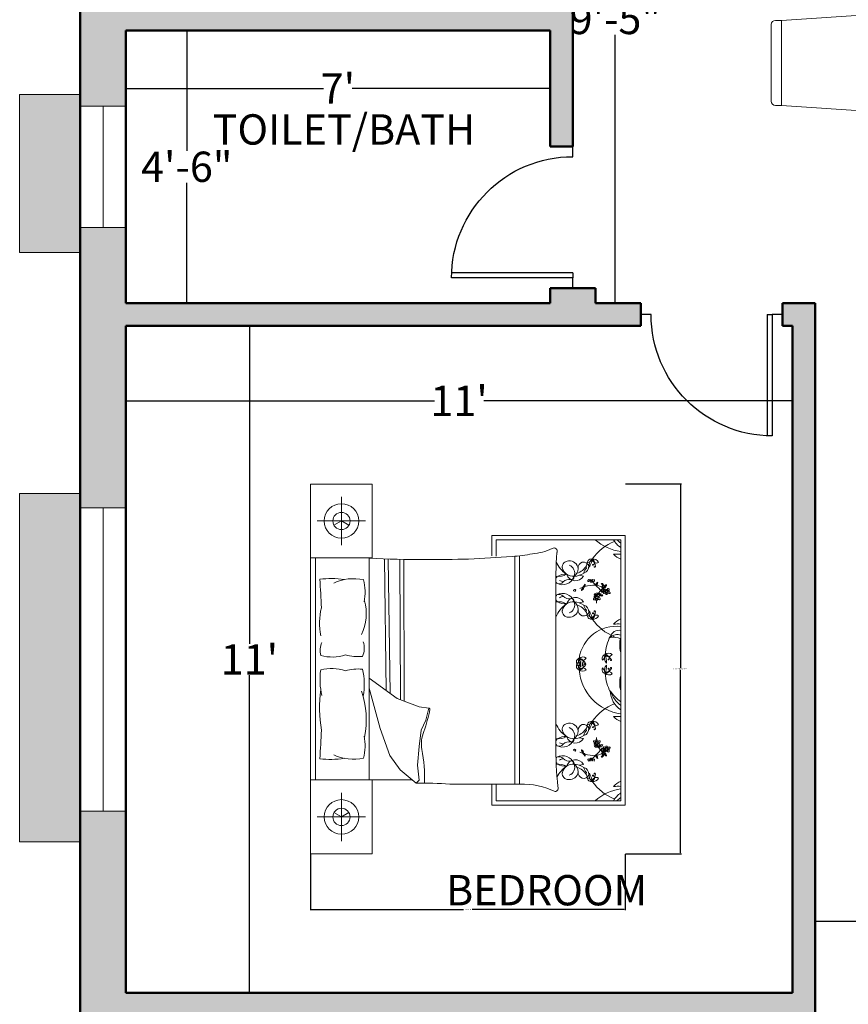
# Model space of a CAD drawing. Units: inches. Extents: x -28 to 544, y -640 to 52.
# Tile 4 of 11: x 5 to 169, y -389 to -194. Entities that reach past the tile are written whole.
import ezdxf

# ---------------------------------------------------------------- set-up
doc = ezdxf.new("R2010")
doc.units = ezdxf.units.IN
doc.header["$MEASUREMENT"] = 0
for name, color, linetype, lineweight in [('A-ANNO-DIMS', 2, 'Continuous', 18), ('A-AREA-IDEN', 7, 'Continuous', 25), ('A-DOOR', 3, 'Continuous', 25), ('A-FURN', 8, 'Continuous', 18), ('A-GLAZ', 4, 'Continuous', 20), ('A-ROOF', 8, 'Continuous', 18), ('A-ROOF-PATT', 252, 'Continuous', 13), ('A-WALL', 7, 'Continuous', 50), ('A-WALL-PATT', 5, 'Continuous', 13)]:
    doc.layers.add(name, color=color, linetype=linetype, lineweight=lineweight)
doc.styles.get("Standard").update_dxf_attribs({"font": 'arial.ttf'})
doc.dimstyles.get("Standard").update_dxf_attribs({"dimtxt": 0.18, "dimasz": 0.18, "dimexe": 0.18, "dimexo": 0.0625, "dimgap": 0.09, "dimtad": 0, "dimtih": 1, "dimtoh": 1, "dimdec": 0, "dimzin": 0, "dimdsep": 46, "dimlunit": 3, "dimtxsty": 'Standard', "dimcen": 0.09, "dimadec": 0, "dimazin": 0, "dimtfac": 1, "dimtdec": 0, "dimtofl": 0, "dimtmove": 0, "dimatfit": 3, "dimfxl": 1, "dimtolj": 1, "dimtzin": 0, "dimarcsym": 0})

# ---------------------------------------------------------------- blocks, each defined once
blk = doc.blocks.new('*D13')
at = {"layer": 'A-ANNO-DIMS', "color": 0, "lineweight": -2, "transparency": 16777216}
for p, q in [((38.26, -196.24), (37.84, -196.24)), ((38.02, -196.42), (38.02, -220.09)), ((38.02, -250.06), (38.02, -226.39)), ((43.05, -250.24), (37.84, -250.24))]:
    blk.add_line(p, q, dxfattribs=at)
at = {"layer": 'A-ANNO-DIMS', "color": 0, "transparency": 16777216}
for points in [[(37.99, -196.42), (38.05, -196.42), (38.02, -196.24)], [(37.99, -250.06), (38.05, -250.06), (38.02, -250.24)]]:
    blk.add_solid(points, dxfattribs=at)
at = {"layer": 'Defpoints', "color": 0, "transparency": 16777216}
for p in [(38.32, -196.24), (38.02, -250.24), (43.11, -250.24)]:
    blk.add_point(p, dxfattribs=at)
at = {"layer": 'A-ANNO-DIMS', "color": 0, "transparency": 16777216, "insert": (38.02, -223.24), "char_height": 6, "attachment_point": 5}
blk.add_mtext('\\A1;4\'-6"', dxfattribs=at)
blk = doc.blocks.new('*D14')
at = {"layer": 'A-ANNO-DIMS', "color": 0, "lineweight": -2, "transparency": 16777216}
for p, q in [((25.94, -207.68), (25.94, -207.56)), ((26.12, -207.74), (65.12, -207.74)), ((109.76, -207.74), (70.77, -207.74)), ((109.94, -207.68), (109.94, -207.56))]:
    blk.add_line(p, q, dxfattribs=at)
at = {"layer": 'A-ANNO-DIMS', "color": 0, "transparency": 16777216}
for points in [[(26.12, -207.71), (26.12, -207.77), (25.94, -207.74)], [(109.76, -207.71), (109.76, -207.77), (109.94, -207.74)]]:
    blk.add_solid(points, dxfattribs=at)
at = {"layer": 'Defpoints', "color": 0, "transparency": 16777216}
for p in [(25.94, -207.74), (25.94, -207.74), (109.94, -207.74)]:
    blk.add_point(p, dxfattribs=at)
at = {"layer": 'A-ANNO-DIMS', "color": 0, "transparency": 16777216, "insert": (67.94, -207.74), "char_height": 6, "attachment_point": 5}
blk.add_mtext("\\A1;7'", dxfattribs=at)
blk = doc.blocks.new('*D15')
at = {"layer": 'A-ANNO-DIMS', "color": 0, "lineweight": -2, "transparency": 16777216}
for p, q in [((50.43, -254.92), (50.43, -317.64)), ((50.5, -254.74), (50.61, -254.74)), ((50.43, -386.56), (50.43, -323.84)), ((50.5, -386.74), (50.61, -386.74))]:
    blk.add_line(p, q, dxfattribs=at)
at = {"layer": 'A-ANNO-DIMS', "color": 0, "transparency": 16777216}
for points in [[(50.4, -254.92), (50.46, -254.92), (50.43, -254.74)], [(50.4, -386.56), (50.46, -386.56), (50.43, -386.74)]]:
    blk.add_solid(points, dxfattribs=at)
at = {"layer": 'Defpoints', "color": 0, "transparency": 16777216}
for p in [(50.43, -254.74), (50.43, -386.74), (50.43, -386.74)]:
    blk.add_point(p, dxfattribs=at)
at = {"layer": 'A-ANNO-DIMS', "color": 0, "transparency": 16777216, "insert": (50.43, -320.74), "char_height": 6, "attachment_point": 5}
blk.add_mtext("\\A1;11'", dxfattribs=at)
blk = doc.blocks.new('*D16')
at = {"layer": 'A-ANNO-DIMS', "color": 0, "lineweight": -2, "transparency": 16777216}
for p, q in [((25.94, -269.5), (25.94, -269.38)), ((26.12, -269.56), (87.05, -269.56)), ((157.76, -269.56), (96.84, -269.56)), ((157.94, -269.5), (157.94, -269.38))]:
    blk.add_line(p, q, dxfattribs=at)
at = {"layer": 'A-ANNO-DIMS', "color": 0, "transparency": 16777216}
for points in [[(26.12, -269.53), (26.12, -269.59), (25.94, -269.56)], [(157.76, -269.53), (157.76, -269.59), (157.94, -269.56)]]:
    blk.add_solid(points, dxfattribs=at)
at = {"layer": 'Defpoints', "color": 0, "transparency": 16777216}
for p in [(25.94, -269.56), (25.94, -269.56), (157.94, -269.56)]:
    blk.add_point(p, dxfattribs=at)
at = {"layer": 'A-ANNO-DIMS', "color": 0, "transparency": 16777216, "insert": (91.94, -269.56), "char_height": 6, "attachment_point": 5}
blk.add_mtext("\\A1;11'", dxfattribs=at)
blk = doc.blocks.new('*D35')
at = {"layer": 'A-ANNO-DIMS', "color": 0, "lineweight": -2, "transparency": 16777216}
for p, q in [((126.88, -137.74), (122.68, -137.74)), ((122.86, -137.92), (122.86, -190.84)), ((122.86, -250.06), (122.86, -197.14)), ((127.88, -250.24), (122.68, -250.24))]:
    blk.add_line(p, q, dxfattribs=at)
at = {"layer": 'A-ANNO-DIMS', "color": 0, "transparency": 16777216}
for points in [[(122.83, -137.92), (122.89, -137.92), (122.86, -137.74)], [(122.83, -250.06), (122.89, -250.06), (122.86, -250.24)]]:
    blk.add_solid(points, dxfattribs=at)
at = {"layer": 'Defpoints', "color": 0, "transparency": 16777216}
for p in [(126.94, -137.74), (122.86, -250.24), (127.94, -250.24)]:
    blk.add_point(p, dxfattribs=at)
at = {"layer": 'A-ANNO-DIMS', "color": 0, "transparency": 16777216, "insert": (122.86, -193.99), "char_height": 6, "attachment_point": 5}
blk.add_mtext('\\A1;9\'-5"', dxfattribs=at)
blk = doc.blocks.new('*D39')
at = {"layer": 'A-ANNO-DIMS', "color": 0, "lineweight": -2, "transparency": 16777216}
for p, q in [((162.44, -377.5), (162.44, -372.33)), ((162.62, -372.51), (201.62, -372.51)), ((246.26, -372.51), (207.27, -372.51)), ((246.44, -377.5), (246.44, -372.33))]:
    blk.add_line(p, q, dxfattribs=at)
at = {"layer": 'A-ANNO-DIMS', "color": 0, "transparency": 16777216}
for points in [[(162.62, -372.48), (162.62, -372.54), (162.44, -372.51)], [(246.26, -372.48), (246.26, -372.54), (246.44, -372.51)]]:
    blk.add_solid(points, dxfattribs=at)
at = {"layer": 'Defpoints', "color": 0, "transparency": 16777216}
for p in [(246.44, -372.51), (162.44, -377.56), (246.44, -377.56)]:
    blk.add_point(p, dxfattribs=at)
at = {"layer": 'A-ANNO-DIMS', "color": 0, "transparency": 16777216, "insert": (204.44, -372.51), "char_height": 6, "attachment_point": 5}
blk.add_mtext("\\A1;7'", dxfattribs=at)
blk = doc.blocks.new('BED-DOUBLE-HEADBOARD-73')
for p, q in [((0, 0), (0, 73.21)), ((6.1, 61.11), (6.1, 70.67)), ((10.88, 65.89), (1.32, 65.89)), ((35.89, 58.98), (35.89, 63.04)), ((35.89, 63.04), (62.26, 63.04)), ((62.26, 63.04), (62.26, 9.66)), ((36.74, 62.19), (36.74, 58.96)), ((61.41, 62.19), (36.74, 62.19)), ((61.41, 10.51), (61.41, 62.19)), ((0.94, 58.57), (0.94, 14.64)), ((11.57, 14.64), (11.57, 58.57)), ((40.45, 58.9), (40.45, 13.8)), ((41.37, 58.97), (41.37, 13.8)), ((14.61, 58.37), (14.98, 32.31)), ((15.36, 58.34), (15.74, 31.76)), ((17.67, 58.31), (17.78, 30.51)), ((18.42, 58.31), (18.53, 30.22)), ((53.99, 54.97), (53.16, 55.14)), ((48.56, 51.47), (48.56, 21.74)), ((53.99, 49.86), (53.16, 49.7)), ((11.57, 34.76), (17.15, 30.74)), ((13.75, 24.81), (11.57, 32.8)), ((17.15, 30.74), (21.45, 29.11)), ((21.45, 29.11), (23.38, 28.82)), ((23.38, 28.82), (22.79, 26.44)), ((22.79, 26.44), (21.9, 24.52)), ((15.67, 19.47), (13.75, 24.81)), ((21.9, 24.52), (21.45, 21.25)), ((53.99, 22.84), (53.16, 23)), ((21.45, 21.25), (21.15, 17.55)), ((17.75, 16.66), (15.67, 19.47)), ((21.15, 17.55), (21.45, 14.58)), ((53.99, 17.73), (53.16, 17.56)), ((20.86, 13.99), (17.75, 16.66)), ((0, 14.64), (20.09, 14.64)), ((21.45, 14.58), (20.86, 13.99)), ((35.89, 9.66), (35.89, 13.8)), ((36.74, 13.8), (36.74, 10.51)), ((6.1, 12.1), (6.1, 2.54)), ((36.74, 10.51), (61.41, 10.51)), ((62.26, 9.66), (35.89, 9.66)), ((10.88, 7.32), (1.32, 7.32))]:
    blk.add_line(p, q)
for points in [[(0, 58.57), (12.2, 58.57), (12.2, 73.21), (0, 73.21)], [(6.1, 65.89), (4.62, 65.04)], [(6.1, 65.89), (7.58, 65.04)], [(12.2, 14.64), (12.2, 0), (0, 0)], [(6.1, 7.32), (4.62, 8.18)], [(6.1, 7.32), (7.58, 8.18)]]:
    blk.add_lwpolyline(points)
for points in [[(39.88, 58.88, 0.056112), (43.91, 59.41, 0.095341), (47.79, 60.44)], [(1.82, 54.36, -0.074897), (6.61, 54.28, 0.472817)], [(6.87, 39.39, -0.14099), (2, 39.24, -0.235245)], [(6.87, 36.26, 0.14099), (2, 36.41, 0.235245)], [(1.82, 18.85, 0.074897), (6.61, 18.94, -0.472817)], [(27.56, 13.83, 0.001242), (41.45, 13.8, -0.127202), (48.38, 12.33)]]:
    blk.add_lwpolyline(points, format="xyb")
for centre, radius in [((6.1, 65.89), 3.42), ((6.1, 65.89), 1.71), ((56.64, 50.74), 0.186), ((58.61, 51.96), 0.186), ((56.64, 21.96), 0.186), ((58.61, 20.74), 0.186), ((6.1, 7.32), 3.42), ((6.1, 7.32), 1.71)]:
    blk.add_circle(centre, radius)
for centre, radius, start, end in [((48.16, 59.89), 0.667, 336.5219, 123.8264), ((63.65, 52.95), 9.56, 111.4092, 145.6135), ((62.7, 69.31), 9.56, 228.1144, 262.255), ((63.98, 64.51), 4.66, 209.8884, 236.5383), ((64.85, 66.19), 5.81, 223.5186, 233.6964), ((20.52, 189.81), 131.55, 266.1, 270.9282), ((25.3, 229.86), 171.6, 269.1145, 274.8735), ((119.76, 53.71), 71.24, 175.2402, 181.8035), ((62.9, 61.9), 3.89, 221.0454, 247.4453), ((60.81, 72.55), 13.23, 266.3481, 272.5919), ((53.71, 59.98), 5.54, 203.6453, 236.3329), ((51.05, 56.75), 1.24, 88.9462, 185.5144), ((51.97, 57.13), 2.2, 193.079, 274.7067), ((51.23, 56.25), 1.75, 7.1143, 95.0551), ((50.57, 55.56), 1.7, 338.5779, 68.4181), ((51.63, 58.83), 3.46, 288.2955, 328.7386), ((54.05, 56.65), 1.1, 19.1312, 189.736), ((53.72, 56.91), 1.37, 285.6955, 4.031), ((55.54, 55.43), 1.46, 128.4175, 173.8338), ((55.24, 56.88), 0.673, 126.7319, 206.0245), ((55.57, 57.58), 0.793, 76.272, 177.0484), ((54.36, 59.2), 1.63, 284.7031, 328.6173), ((56.64, 57.12), 1.51, 125.7657, 194.5347), ((49.23, 59.8), 6.69, 332.8176, 347.4827), ((55.98, 57.31), 1.06, 20.9613, 102.2885), ((56.55, 58.37), 0.798, 181.7131, 301.5367), ((53.94, 56.76), 2.42, 2.0648, 41.1598), ((55.39, 57.66), 0.782, 316.2238, 62.3173), ((55.84, 57.2), 0.0623, 20.2667, 316.2271), ((56.17, 56.85), 0.0577, 52.0591, 168.5166), ((56.23, 56.84), 0.119, 168.5166, 2.0648), ((49.1, 57.95), 3.03, 259.249, 301.1782), ((49.37, 54.19), 0.882, 127.675, 162.5814), ((49.89, 55.6), 2.33, 240.8249, 340.7178), ((50.42, 52.56), 2.82, 85.2696, 124.215), ((52.41, 55.88), 1.82, 196.8663, 330.0915), ((51.65, 54.73), 0.454, 254.8529, 12.6959), ((50.42, 52.56), 2.82, 53.6555, 57.2989), ((50.84, 56.55), 2.13, 305.9599, 357.6409), ((51.91, 58.86), 3.93, 273.4924, 303.7117), ((-694.9, 14.01), 697.9, 2.85022, 3.31479), ((8.53, 45.04), 9.44, 78.2417, 114.8684), ((0.97, 51.75), 9.81, 348.9631, 14.8961), ((49.37, 54.19), 0.882, 196.6343, 225.5483), ((49.19, 54.56), 1.1, 246.1646, 318.4347), ((50.31, 55.95), 2.1, 240.0851, 262.564), ((51.14, 52.84), 1.5, 74.8529, 138.4347), ((56.02, 47.13), 6.06, 110.1059, 116.9968), ((53.95, 52.6), 0.149, 83.9457, 185.6216), ((53.35, 52.74), 0.614, 328.836, 0.8141), ((53.67, 52.56), 0.351, 306.5232, 32.4668), ((54.09, 52.83), 0.149, 112.5583, 214.2343), ((53.99, 53.1), 0.351, 265.7131, 351.6568), ((53.68, 53.29), 0.614, 297.3659, 329.344), ((53.22, 53.82), 1.18, 313.6929, 321.7899), ((54.52, 53.01), 0.384, 115.5379, 168.6744), ((53.21, 53.57), 1.16, 329.344, 349.7412), ((56.02, 47.13), 6.06, 86.1723, 106.4158), ((52.29, 53.3), 2.06, 352.8698, 1.6736), ((55.02, 54.05), 0.144, 125.0752, 284.7644), ((55.25, 54.1), 0.311, 127.3642, 168.4363), ((55, 54.35), 0.448, 277.4968, 341.2737), ((55.36, 54.14), 0.178, 88.1325, 178.8919), ((55.72, 53.95), 0.385, 136.3462, 189.6513), ((55.5, 53.92), 0.161, 189.6513, 312.3208), ((55.54, 54.36), 0.186, 183.2768, 356.7232), ((56.12, 54.03), 0.61, 164.2829, 186.9148), ((55.4, 54.02), 0.305, 312.3208, 40.2111), ((56.04, 54.37), 0.433, 201.6382, 274.947), ((55.47, 53.77), 0.566, 42.3896, 66.5724), ((61.18, 58.25), 6.95, 217.9541, 226.8459), ((55.88, 54.11), 0.308, 10.9597, 52.2379), ((56.07, 54.08), 0.143, 274.947, 37.5263), ((56.55, 53.27), 0.149, 112.5583, 214.2343), ((56.45, 53.53), 0.351, 265.7131, 351.6568), ((56.14, 53.73), 0.614, 297.3659, 329.344), ((56.17, 50.15), 3.04, 60.7959, 85.244), ((49.7, 45.78), 10, 37.8256, 47.7588), ((55.68, 54.25), 1.18, 313.6929, 321.7899), ((56.98, 53.45), 0.384, 115.5379, 168.6744), ((55.68, 54), 1.16, 329.344, 349.7412), ((54.75, 53.74), 2.06, 352.8698, 1.6736), ((60.21, 49.84), 3.65, 130.182, 149.456), ((57.66, 53.32), 0.208, 33.0979, 123.1364), ((53.07, 50.39), 5.45, 31.1156, 34.8118), ((57.35, 52.96), 0.564, 2.3172, 70.5201), ((57.08, 52.35), 0.85, 310.9365, 22.7695), ((57.82, 52.83), 0.163, 135.7354, 318.1297), ((57.55, 53.09), 0.216, 315.7354, 31.1156), ((57.37, 52.63), 0.5, 319.3812, 5.5456), ((57.94, 52.83), 0.163, 68.2452, 250.6395), ((57.57, 53.03), 0.485, 352.6008, 57.1845), ((59.3, 49.77), 3.25, 111.7087, 116.2181), ((56.17, 50.15), 3.04, 47.5083, 55.9967), ((58.03, 53.14), 0.485, 252.8042, 349.6943), ((57.57, 52.27), 0.517, 331.1838, 51.6792), ((58.08, 53.18), 0.216, 248.2452, 323.6254), ((57.89, 53.31), 0.564, 291.7087, 3.0299), ((53.87, 56.28), 5.45, 323.6254, 327.3216), ((58.34, 53.17), 0.208, 325.6077, 55.6462), ((49.37, 50.64), 0.882, 134.4517, 156.7144), ((49.89, 49.23), 2.33, 19.2822, 119.1751), ((49.19, 50.27), 1.1, 41.5653, 113.8354), ((50.31, 48.88), 2.1, 97.436, 119.9149), ((51.14, 51.99), 1.5, 221.5653, 285.1471), ((52.41, 48.95), 1.82, 29.9085, 163.1337), ((52.25, 52.22), 0.229, 169.5864, 349.5616), ((52.34, 52.21), 0.141, 349.5616, 167.2949), ((53.99, 52.13), 0.384, 129.5056, 182.6421), ((52.88, 53.02), 1.16, 308.4388, 328.836), ((52.68, 53.96), 2.06, 296.5064, 305.3102), ((52.67, 52.9), 1.18, 336.3901, 344.4871), ((56.35, 50.49), 0.311, 93.635, 168.4363), ((56.37, 52.17), 0.85, 253.6301, 325.4631), ((56.6, 50.99), 0.601, 82.0748, 142.6895), ((56.54, 51.82), 0.617, 228.342, 274.9894), ((56.31, 50.98), 0.183, 138.2946, 276.2474), ((56.38, 50.95), 0.254, 358.5719, 143.8954), ((56.47, 50.53), 0.178, 88.1325, 178.8919), ((56.53, 51.15), 0.257, 208.8493, 269.9355), ((56.31, 51.09), 0.293, 274.2123, 318.1587), ((56.56, 51.72), 0.517, 273.8774, 357.1501), ((57.21, 50.79), 0.588, 121.9501, 165.2442), ((56.76, 52.08), 0.5, 262.0748, 308.2393), ((56.8, 51.02), 0.123, 262.868, 7.094), ((56.58, 50.16), 0.566, 42.3896, 66.5724), ((56.79, 51.12), 0.368, 278.5614, 22.5914), ((56.99, 50.49), 0.308, 10.9597, 118.7804), ((60.21, 49.84), 3.65, 156.1523, 156.9499), ((56.99, 51.14), 0.185, 44.3732, 121.9501), ((57.56, 51.57), 0.517, 181.4625, 249.4747), ((57.48, 51.98), 0.5, 215.1128, 261.2773), ((57.88, 51.95), 0.85, 197.889, 269.722), ((57.61, 51.66), 0.617, 248.3627, 295.0101), ((57.31, 50.89), 0.601, 20.6625, 81.2773), ((58.2, 51.92), 0.601, 139.3812, 199.9959), ((57.47, 52.31), 0.617, 285.6484, 332.2957), ((58.1, 51.65), 0.144, 125.0752, 284.7644), ((58.32, 51.71), 0.311, 93.635, 168.4363), ((58.28, 52.2), 0.183, 138.2946, 276.2474), ((58.08, 51.96), 0.448, 277.4968, 341.2737), ((58.35, 52.17), 0.254, 358.5719, 143.8954), ((58.43, 51.75), 0.178, 88.1325, 178.8919), ((58.5, 52.37), 0.257, 208.8493, 269.9355), ((58.28, 52.31), 0.293, 274.2123, 318.1587), ((58.79, 51.56), 0.385, 136.3462, 189.6513), ((58.57, 51.52), 0.161, 189.6513, 312.3208), ((59.19, 51.63), 0.61, 164.2829, 186.9148), ((59.17, 52.01), 0.588, 121.9501, 165.2442), ((58.47, 51.63), 0.305, 312.3208, 40.2111), ((59.12, 51.97), 0.433, 201.6382, 274.947), ((58.77, 52.24), 0.123, 262.868, 7.094), ((58.54, 51.38), 0.566, 42.3896, 66.5724), ((58.75, 52.34), 0.368, 278.5614, 22.5914), ((58.95, 51.71), 0.308, 10.9597, 118.7804), ((58.96, 52.36), 0.185, 44.3732, 121.9501), ((59.14, 51.68), 0.143, 274.947, 37.5263), ((1.69, 47.52), 9.32, 333.8761, 16.1746), ((49.37, 50.64), 0.882, 203.2856, 232.325), ((49.1, 46.88), 3.03, 58.8218, 100.2867), ((53.71, 44.85), 5.54, 123.6671, 158.5059), ((50.42, 52.28), 2.82, 235.785, 274.7304), ((51.97, 47.7), 2.2, 85.2933, 166.921), ((50.57, 49.27), 1.7, 291.5819, 21.4221), ((51.65, 50.1), 0.454, 347.3041, 105.1471), ((50.42, 52.28), 2.82, 302.7011, 306.3445), ((50.84, 48.28), 2.13, 2.3591, 54.0401), ((51.91, 45.97), 3.93, 56.2883, 86.5076), ((51.63, 46), 3.46, 31.2614, 71.7045), ((55.54, 49.4), 1.46, 186.1662, 231.5825), ((53.72, 47.92), 1.37, 355.969, 74.3045), ((56.13, 50.43), 0.144, 125.0752, 284.7644), ((56.11, 50.74), 0.448, 277.4968, 341.2737), ((56.83, 50.34), 0.385, 136.3462, 189.6513), ((56.6, 50.3), 0.161, 189.6513, 312.3208), ((60.21, 49.84), 3.65, 175.2415, 182.8929), ((57.23, 50.41), 0.61, 164.2829, 186.9148), ((56.51, 50.41), 0.305, 312.3208, 40.2111), ((57.15, 50.75), 0.433, 201.6382, 274.947), ((57.18, 50.46), 0.143, 274.947, 37.5263), ((14.63, 45.68), 12.87, 166.3427, 191.1841), ((51.05, 48.08), 1.24, 174.4856, 271.0538), ((51.23, 48.59), 1.75, 264.9449, 352.8857), ((54.05, 48.18), 1.1, 170.264, 340.8688), ((55.24, 47.96), 0.673, 153.9755, 233.2681), ((55.57, 47.25), 0.793, 182.9516, 283.728), ((54.36, 45.63), 1.63, 31.3827, 75.2969), ((56.64, 47.71), 1.51, 165.4653, 234.2343), ((49.23, 45.03), 6.69, 12.5173, 27.1824), ((53.94, 48.07), 2.42, 318.8402, 357.9352), ((55.39, 47.18), 0.782, 297.6827, 43.7762), ((56.55, 46.46), 0.798, 58.4633, 178.2869), ((55.98, 47.52), 1.06, 257.7115, 339.0387), ((55.88, 47.64), 0.103, 43.7762, 339.7183), ((56.23, 47.99), 0.119, 357.9352, 191.4834), ((56.17, 47.98), 0.0577, 191.4834, 307.9409), ((60.49, 37.66), 7.4, 82.8636, 171.8197), ((63.65, 51.88), 9.56, 214.3865, 248.5908), ((62.9, 42.93), 3.89, 112.5547, 138.9546), ((60.81, 32.28), 13.23, 87.4081, 93.6519), ((67.82, 38.7), 9.56, 152.5854, 175.5377), ((61.01, 42.54), 1.72, 76.3898, 169.0739), ((60.77, 41.25), 2.17, 72.8609, 131.9049), ((59.82, 38.61), 4.28, 68.117, 96.6195), ((66.44, 41.37), 5.26, 162.9798, 196.4569), ((5.48, 40.25), 3.62, 153.3437, 196.1026), ((6.74, 40.74), 3.88, 335.0183, 18.5407), ((9.32, 48.02), 8.97, 254.1707, 275.9871), ((53.88, 37.92), 1.06, 50.8855, 132.2127), ((58.51, 38.68), 0.793, 106.1963, 206.9726), ((56.66, 39.48), 1.63, 314.6273, 358.5415), ((59.67, 38.82), 1.51, 155.6899, 224.4589), ((59, 38.66), 1.06, 50.8855, 132.2127), ((58.97, 39.86), 0.798, 211.6373, 331.4609), ((57.51, 37.15), 2.42, 31.989, 71.0841), ((51.91, 37.44), 6.69, 2.7418, 17.407), ((58.32, 38.66), 0.782, 346.148, 92.2415), ((69.15, 39.29), 7.77, 174.3643, 175.6213), ((74.47, 35.19), 13.89, 160.0972, 160.2783), ((53.39, 37.95), 0.793, 106.1963, 206.9726), ((53.39, 37.19), 0.793, 153.0274, 253.8037), ((51.54, 38.75), 1.63, 314.6273, 358.5415), ((51.54, 36.39), 1.63, 1.4585, 45.3727), ((54.55, 38.09), 1.51, 155.6899, 224.4589), ((54.55, 37.05), 1.51, 135.5411, 204.3101), ((53.85, 39.13), 0.798, 211.6373, 331.4609), ((53.2, 37.93), 0.782, 346.148, 92.2415), ((52.39, 36.42), 2.42, 31.989, 71.0841), ((46.79, 36.71), 6.69, 2.7418, 17.407), ((46.79, 38.43), 6.69, 342.593, 357.2582), ((52.39, 38.72), 2.42, 288.9159, 328.011), ((53.2, 37.21), 0.782, 267.7585, 13.852), ((53.82, 37.76), 0.0623, 50.1909, 346.0209), ((53.86, 37.38), 0.103, 13.852, 309.9245), ((54.34, 37.64), 0.119, 198.4408, 31.989), ((54.28, 37.62), 0.0577, 81.9833, 198.4408), ((54.34, 37.5), 0.119, 328.011, 161.5592), ((54.28, 37.52), 0.0577, 161.5592, 278.0167), ((59.67, 36.32), 1.51, 135.5411, 204.3101), ((51.91, 37.7), 6.69, 342.593, 357.2582), ((58.94, 38.49), 0.0623, 50.1909, 346.0209), ((59.46, 38.37), 0.119, 198.4408, 31.989), ((59.4, 38.35), 0.0577, 81.9833, 198.4408), ((14.9, 34.49), 13.05, 171.5249, 193.96), ((9.32, 27.63), 8.97, 84.0129, 105.8293), ((-2.29, 33.51), 12.91, 349.8617, 13.6238), ((53.85, 36.01), 0.798, 28.5391, 148.3627), ((53.88, 37.22), 1.06, 227.7873, 309.1145), ((62.7, 37.18), 9.56, 184.4623, 262.255), ((58.51, 36.46), 0.793, 153.0274, 253.8037), ((56.66, 35.66), 1.63, 1.4585, 45.3727), ((57.51, 37.99), 2.42, 288.9159, 328.011), ((58.32, 36.48), 0.782, 267.7585, 13.852), ((58.97, 35.28), 0.798, 28.5391, 148.3627), ((59, 36.48), 1.06, 227.7873, 309.1145), ((67.82, 36.44), 9.56, 184.4623, 207.4146), ((58.98, 36.64), 0.103, 13.852, 309.9245), ((59.46, 36.77), 0.119, 328.011, 161.5592), ((59.4, 36.79), 0.0577, 161.5592, 278.0167), ((66.44, 33.77), 5.26, 163.5431, 197.0202), ((69.15, 35.85), 7.77, 184.3787, 185.6357), ((74.47, 39.95), 13.89, 199.7217, 199.9028), ((28.32, 28.88), 26.55, 172.2196, 189.497), ((-6.01, 26.62), 17.02, 348.0397, 19.2615), ((63.98, 32.38), 4.66, 181.272, 236.5383), ((66.48, 37.11), 8.64, 214.0123, 234.053), ((64.85, 34.06), 5.81, 197.8504, 233.6964), ((63.65, 20.82), 9.56, 111.4092, 145.6135), ((-4.29, 33.9), 28.39, 340.1194, 349.3383), ((23.44, 28.65), 0.177, 358.8623, 109.7536), ((53.71, 27.85), 5.54, 201.4941, 236.3329), ((51.05, 24.62), 1.24, 88.9462, 185.5144), ((51.23, 24.12), 1.75, 7.1143, 95.0551), ((54.05, 24.52), 1.1, 19.1312, 189.736), ((55.57, 25.45), 0.793, 76.272, 177.0484), ((54.36, 27.07), 1.63, 284.7031, 328.6173), ((56.64, 24.99), 1.51, 125.7657, 194.5347), ((49.23, 27.67), 6.69, 332.8176, 347.4827), ((55.98, 25.18), 1.06, 20.9613, 102.2885), ((55.39, 25.53), 0.782, 316.2238, 62.3173), ((53.94, 24.63), 2.42, 2.0648, 41.1598), ((56.55, 26.24), 0.798, 181.7131, 301.5367), ((60.81, 40.42), 13.23, 266.3481, 272.5919), ((62.9, 29.77), 3.89, 221.0454, 247.4453), ((-694.9, 59.2), 697.9, 356.68521, 357.14978), ((27.87, 21.84), 5.96, 156.2616, 191.3392), ((51.97, 25), 2.2, 193.079, 274.7067), ((50.57, 23.43), 1.7, 338.5779, 68.4181), ((50.84, 24.42), 2.13, 305.9599, 357.6409), ((51.91, 26.73), 3.93, 273.4924, 303.7117), ((51.63, 26.7), 3.46, 288.2955, 328.7386), ((53.72, 24.78), 1.37, 285.6955, 4.031), ((55.54, 23.3), 1.46, 128.4175, 173.8338), ((55.24, 24.74), 0.673, 126.7319, 206.0245), ((55.84, 25.07), 0.0623, 20.2667, 316.2271), ((56.17, 24.72), 0.0577, 52.0591, 168.5166), ((56.23, 24.71), 0.119, 168.5166, 2.0648), ((0.97, 21.46), 9.81, 345.1039, 11.0369), ((124.77, 20.87), 76.21, 179.3433, 185.6887), ((49.1, 25.82), 3.03, 259.7133, 301.1782), ((49.37, 22.06), 0.882, 127.675, 156.7144), ((49.37, 22.06), 0.882, 203.229, 225.5483), ((49.89, 23.47), 2.33, 240.8249, 340.7178), ((49.19, 22.43), 1.1, 246.1646, 318.4347), ((50.42, 20.42), 2.82, 85.2696, 124.215), ((50.31, 23.82), 2.1, 240.0851, 262.564), ((51.14, 20.71), 1.5, 74.8529, 138.4347), ((52.41, 23.75), 1.82, 196.8663, 330.0915), ((51.65, 22.6), 0.454, 254.8529, 12.6959), ((50.42, 20.42), 2.82, 53.6555, 57.2989), ((56.13, 22.27), 0.144, 75.2356, 234.9248), ((56.35, 22.21), 0.311, 191.5637, 266.365), ((56.31, 21.72), 0.183, 83.7526, 221.7054), ((56.54, 20.88), 0.617, 85.0106, 131.658), ((56.11, 21.96), 0.448, 18.7263, 82.5032), ((56.38, 21.75), 0.254, 216.1046, 1.4281), ((56.47, 22.17), 0.178, 181.1081, 271.8675), ((56.53, 21.55), 0.257, 90.0645, 151.1507), ((56.31, 21.61), 0.293, 41.8413, 85.7877), ((56.83, 22.36), 0.385, 170.3487, 223.6538), ((56.6, 22.4), 0.161, 47.6792, 170.3487), ((60.21, 22.86), 3.65, 177.1071, 184.7585), ((56.56, 20.98), 0.517, 2.8499, 86.1226), ((57.23, 22.29), 0.61, 173.0852, 195.7171), ((57.21, 21.91), 0.588, 194.7558, 238.0499), ((56.51, 22.29), 0.305, 319.7889, 47.6792), ((57.15, 21.95), 0.433, 85.053, 158.3618), ((56.8, 21.68), 0.123, 352.906, 97.132), ((56.58, 22.54), 0.566, 293.4276, 317.6104), ((56.99, 22.21), 0.308, 241.2196, 349.0403), ((56.79, 21.58), 0.368, 337.4086, 81.4386), ((56.99, 21.56), 0.185, 238.0499, 315.6268), ((57.56, 21.13), 0.517, 110.5253, 178.5375), ((57.88, 20.75), 0.85, 90.278, 162.111), ((57.18, 22.24), 0.143, 322.4737, 85.053), ((57.61, 21.04), 0.617, 64.9899, 111.6373), ((57.31, 21.81), 0.601, 278.7227, 339.3375), ((8.53, 28.17), 9.44, 245.1316, 281.7583), ((-5.07, 15.24), 27.63, 357.4519, 11.3392), ((52.25, 20.48), 0.229, 10.4384, 190.4136), ((52.34, 20.49), 0.141, 192.7051, 10.4384), ((56.02, 25.57), 6.06, 243.0032, 249.8941), ((52.88, 19.68), 1.16, 31.164, 51.5612), ((53.99, 20.57), 0.384, 177.3579, 230.4944), ((52.68, 18.74), 2.06, 54.6898, 63.4936), ((52.67, 19.8), 1.18, 15.5129, 23.6099), ((53.95, 20.1), 0.149, 174.3784, 276.0543), ((53.35, 19.96), 0.614, 359.1859, 31.164), ((53.67, 20.14), 0.351, 327.5332, 53.4768), ((54.09, 19.87), 0.149, 145.7657, 247.4417), ((53.99, 19.61), 0.351, 8.3432, 94.2869), ((53.68, 19.41), 0.614, 30.656, 62.6341), ((53.22, 18.88), 1.18, 38.2101, 46.3071), ((54.52, 19.69), 0.384, 191.3256, 244.4621), ((53.21, 19.13), 1.16, 10.2588, 30.656), ((56.02, 25.57), 6.06, 253.5842, 273.8277), ((52.29, 19.4), 2.06, 358.3264, 7.1302), ((61.18, 14.45), 6.95, 133.1541, 142.0459), ((56.37, 20.53), 0.85, 34.5369, 106.3699), ((56.6, 21.71), 0.601, 217.3105, 277.9252), ((56.55, 19.44), 0.149, 145.7657, 247.4417), ((49.7, 26.92), 10, 312.2412, 322.1744), ((56.17, 22.55), 3.04, 274.756, 299.2041), ((56.45, 19.17), 0.351, 8.3432, 94.2869), ((56.14, 18.97), 0.614, 30.656, 62.6341), ((56.76, 20.62), 0.5, 51.7607, 97.9252), ((60.21, 22.86), 3.65, 203.0501, 203.8477), ((57.48, 20.72), 0.5, 98.7227, 144.8872), ((60.21, 22.86), 3.65, 210.544, 229.818), ((57.35, 19.74), 0.564, 289.4799, 357.6828), ((53.07, 22.32), 5.45, 325.1882, 328.8844), ((58.2, 20.78), 0.601, 160.0041, 220.6188), ((57.08, 20.35), 0.85, 337.2305, 49.0635), ((57.47, 20.4), 0.617, 27.7043, 74.3516), ((57.82, 19.88), 0.163, 41.8703, 224.2646), ((57.55, 19.61), 0.216, 328.8844, 44.2646), ((57.37, 20.07), 0.5, 354.4544, 40.6188), ((57.94, 19.87), 0.163, 109.3605, 291.7548), ((57.57, 19.67), 0.485, 302.8155, 7.3992), ((56.17, 22.55), 3.04, 304.0033, 312.4917), ((59.3, 22.93), 3.25, 243.7819, 248.2913), ((57.57, 20.43), 0.517, 308.3208, 28.8162), ((58.03, 19.56), 0.485, 10.3057, 107.1958), ((58.1, 21.05), 0.144, 75.2356, 234.9248), ((58.08, 19.52), 0.216, 36.3746, 111.7548), ((58.32, 20.99), 0.311, 191.5637, 266.365), ((58.28, 20.5), 0.183, 83.7526, 221.7054), ((57.89, 19.39), 0.564, 356.9701, 68.2913), ((58.08, 20.74), 0.448, 18.7263, 82.5032), ((58.35, 20.53), 0.254, 216.1046, 1.4281), ((58.43, 20.95), 0.178, 181.1081, 271.8675), ((53.87, 16.42), 5.45, 32.6784, 36.3746), ((58.5, 20.33), 0.257, 90.0645, 151.1507), ((58.28, 20.39), 0.293, 41.8413, 85.7877), ((58.79, 21.14), 0.385, 170.3487, 223.6538), ((58.57, 21.18), 0.161, 47.6792, 170.3487), ((58.34, 19.53), 0.208, 304.3538, 34.3923), ((59.19, 21.07), 0.61, 173.0852, 195.7171), ((59.17, 20.69), 0.588, 194.7558, 238.0499), ((58.47, 21.07), 0.305, 319.7889, 47.6792), ((59.12, 20.73), 0.433, 85.053, 158.3618), ((58.77, 20.46), 0.123, 352.906, 97.132), ((58.54, 21.32), 0.566, 293.4276, 317.6104), ((58.95, 20.99), 0.308, 241.2196, 349.0403), ((58.75, 20.36), 0.368, 337.4086, 81.4386), ((58.96, 20.34), 0.185, 238.0499, 315.6268), ((59.14, 21.02), 0.143, 322.4737, 85.053), ((49.37, 18.51), 0.882, 134.4517, 153.558), ((49.37, 18.51), 0.882, 210.0293, 232.325), ((49.1, 14.75), 3.03, 58.8218, 99.1554), ((49.89, 17.1), 2.33, 19.2822, 119.1751), ((49.19, 18.14), 1.1, 41.5653, 113.8354), ((50.42, 20.15), 2.82, 235.785, 274.7304), ((50.31, 16.75), 2.1, 97.436, 119.9149), ((51.97, 15.57), 2.2, 85.2933, 166.921), ((51.14, 19.86), 1.5, 221.5653, 285.1471), ((52.41, 16.82), 1.82, 29.9085, 163.1337), ((50.57, 17.14), 1.7, 291.5819, 21.4221), ((51.65, 17.97), 0.454, 347.3041, 105.1471), ((50.42, 20.15), 2.82, 302.7011, 306.3445), ((50.84, 16.15), 2.13, 2.3591, 54.0401), ((51.91, 13.84), 3.93, 56.2883, 86.5076), ((55.02, 18.65), 0.144, 75.2356, 234.9248), ((55.25, 18.6), 0.311, 191.5637, 232.6358), ((55, 18.35), 0.448, 18.7263, 82.5032), ((55.36, 18.56), 0.178, 181.1081, 271.8675), ((55.72, 18.75), 0.385, 170.3487, 223.6538), ((55.5, 18.79), 0.161, 47.6792, 170.3487), ((55.54, 18.34), 0.186, 3.2768, 176.7232), ((56.12, 18.67), 0.61, 173.0852, 195.7171), ((55.4, 18.68), 0.305, 319.7889, 47.6792), ((56.04, 18.34), 0.433, 85.053, 158.3618), ((55.47, 18.93), 0.566, 293.4276, 317.6104), ((55.88, 18.6), 0.308, 307.7621, 349.0403), ((56.07, 18.62), 0.143, 322.4737, 85.053), ((55.68, 18.45), 1.18, 38.2101, 46.3071), ((56.98, 19.25), 0.384, 191.3256, 244.4621), ((55.68, 18.7), 1.16, 10.2588, 30.656), ((54.75, 18.96), 2.06, 358.3264, 7.1302), ((57.66, 19.38), 0.208, 236.8636, 326.9021), ((53.71, 12.72), 5.54, 123.6671, 153.2997), ((51.05, 15.95), 1.24, 174.4856, 271.0538), ((51.23, 16.45), 1.75, 264.9449, 352.8857), ((51.63, 13.87), 3.46, 31.2614, 71.7045), ((54.05, 16.05), 1.1, 170.264, 340.8688), ((53.72, 15.79), 1.37, 355.969, 74.3045), ((55.54, 17.27), 1.46, 186.1662, 231.5825), ((55.24, 15.83), 0.673, 153.9755, 233.2681), ((56.64, 15.58), 1.51, 165.4653, 234.2343), ((49.23, 12.9), 6.69, 12.5173, 27.1824), ((53.94, 15.94), 2.42, 318.8402, 357.9352), ((55.88, 15.51), 0.103, 43.7762, 339.7183), ((56.23, 15.86), 0.119, 357.9352, 191.4834), ((56.17, 15.85), 0.0577, 191.4834, 307.9409), ((22.68, -53.14), 67.15, 85.8294, 91.553), ((54.36, 13.5), 1.63, 31.3827, 75.2969), ((55.57, 15.12), 0.793, 182.9516, 283.728), ((55.39, 15.04), 0.782, 297.6827, 43.7762), ((56.55, 14.33), 0.798, 58.4633, 178.2869), ((55.98, 15.39), 1.06, 257.7115, 339.0387), ((63.65, 19.75), 9.56, 214.3865, 248.5908), ((62.9, 10.8), 3.89, 112.5547, 138.9546), ((48.33, 13.01), 0.676, 273.98, 27.3412), ((62.7, 3.39), 9.56, 97.745, 131.8856), ((63.98, 8.19), 4.66, 123.4617, 150.1116), ((60.81, 0.15), 13.23, 87.4081, 93.6519), ((64.85, 6.51), 5.81, 126.3036, 136.4814)]:
    blk.add_arc(centre, radius, start, end)
blk = doc.blocks.new('DINING-SET-4')
for p, q in [((0.82, 49.45), (2.05, 49.45)), ((18.79, 50.59), (2.05, 49.45)), ((2.05, 32.63), (2.05, 49.45)), ((20.52, 48.95), (20.52, 33.13)), ((56.54, 48.95), (56.54, 33.13)), ((58.27, 50.59), (75.01, 49.45)), ((76.24, 49.45), (75.01, 49.45)), ((75.01, 32.63), (75.01, 49.45)), ((0, 33.45), (0, 48.63)), ((77.06, 33.45), (77.06, 48.63)), ((2.05, 32.63), (0.82, 32.63)), ((2.05, 32.63), (18.79, 31.49)), ((75.01, 32.63), (58.27, 31.49)), ((75.01, 32.63), (76.24, 32.63)), ((2.05, 22.09), (0.82, 22.09)), ((2.05, 22.09), (18.79, 23.23)), ((2.05, 22.09), (2.05, 5.27)), ((20.52, 5.77), (20.52, 21.59)), ((56.54, 5.77), (56.54, 21.59)), ((75.01, 22.09), (58.27, 23.23)), ((75.01, 22.09), (76.24, 22.09)), ((75.01, 22.09), (75.01, 5.27)), ((0, 21.27), (0, 6.09)), ((77.06, 21.27), (77.06, 6.09)), ((0.82, 5.27), (2.05, 5.27)), ((18.79, 4.13), (2.05, 5.27)), ((58.27, 4.13), (75.01, 5.27)), ((76.24, 5.27), (75.01, 5.27))]:
    blk.add_line(p, q)
for points in [[(55.63, 0), (21.43, 0), (21.43, 54.72), (55.63, 54.72)], [(53.35, 2.28), (23.71, 2.28), (23.71, 52.44), (53.35, 52.44)]]:
    blk.add_lwpolyline(points, close=True)
for centre, radius, start, end in [((0.82, 48.63), 0.821, 90, 180), ((18.88, 48.95), 1.64, 0, 93.1221), ((58.18, 48.95), 1.64, 86.8779, 180), ((76.24, 48.63), 0.821, 0, 90), ((0.82, 33.45), 0.821, 180, 270), ((18.88, 33.13), 1.64, 266.8779, 0), ((58.18, 33.13), 1.64, 180, 273.1221), ((76.24, 33.45), 0.821, 270, 0), ((0.82, 21.27), 0.821, 90, 180), ((18.88, 21.59), 1.64, 0, 93.1221), ((58.18, 21.59), 1.64, 86.8779, 180), ((76.24, 21.27), 0.821, 0, 90), ((0.82, 6.09), 0.821, 180, 270), ((76.24, 6.09), 0.821, 270, 0), ((18.88, 5.77), 1.64, 266.8779, 0), ((58.18, 5.77), 1.64, 180, 273.1221)]:
    blk.add_arc(centre, radius, start, end)
blk = doc.blocks.new('WIN-60IN')
for p, q in [((0, 9), (60, 9)), ((0, 0), (0, 9)), ((60, 9), (60, 0)), ((0, 4.5), (60, 4.5)), ((60, 0), (0, 0))]:
    blk.add_line(p, q)
blk = doc.blocks.new('WIN-24IN')
for p, q in [((0, 0), (0, 24)), ((0, 24), (9, 24)), ((4.5, 0), (4.5, 24)), ((9, 24), (9, 0)), ((9, 0), (0, 0))]:
    blk.add_line(p, q)
blk = doc.blocks.new('DOOR-SWING-24IN')
for p, q in [((25, 0), (25, 24)), ((26, 0), (26, 24)), ((2, 0), (0, 0)), ((25, 0), (26, 0)), ((28, 0), (26, 0))]:
    blk.add_line(p, q)
blk.add_arc((26, 0), 24, 90, 180)
blk = doc.blocks.new('*D67')
at = {"layer": 'A-ANNO-DIMS', "color": 0, "lineweight": -2, "transparency": 16777216}
for p, q in [((124.87, -286.01), (135.97, -286.01)), ((135.79, -286.19), (135.79, -322.44)), ((135.79, -359.04), (135.79, -322.8)), ((124.87, -359.22), (135.97, -359.22))]:
    blk.add_line(p, q, dxfattribs=at)
at = {"layer": 'A-ANNO-DIMS', "color": 0, "transparency": 16777216}
for points in [[(135.76, -286.19), (135.82, -286.19), (135.79, -286.01)], [(135.76, -359.04), (135.82, -359.04), (135.79, -359.22)]]:
    blk.add_solid(points, dxfattribs=at)
at = {"layer": 'Defpoints', "color": 0, "transparency": 16777216}
for p in [(124.81, -286.01), (135.79, -286.01), (124.81, -359.22)]:
    blk.add_point(p, dxfattribs=at)
at = {"layer": 'A-ANNO-DIMS', "color": 0, "transparency": 16777216, "insert": (135.79, -322.62), "char_height": 0.18, "attachment_point": 5}
blk.add_mtext('\\A1;DOUBLE BED B 6\'-1" TYP.', dxfattribs=at)
blk = doc.blocks.new('*D68')
at = {"layer": 'A-ANNO-DIMS', "color": 0, "lineweight": -2, "transparency": 16777216}
for p, q in [((62.55, -359.29), (62.55, -370.39)), ((124.81, -359.29), (124.81, -370.39)), ((62.73, -370.21), (92.83, -370.21)), ((124.63, -370.21), (94.53, -370.21))]:
    blk.add_line(p, q, dxfattribs=at)
at = {"layer": 'A-ANNO-DIMS', "color": 0, "transparency": 16777216}
for points in [[(62.73, -370.18), (62.73, -370.24), (62.55, -370.21)], [(124.63, -370.18), (124.63, -370.24), (124.81, -370.21)]]:
    blk.add_solid(points, dxfattribs=at)
at = {"layer": 'Defpoints', "color": 0, "transparency": 16777216}
for p in [(62.55, -359.22), (124.81, -359.22), (124.81, -370.21)]:
    blk.add_point(p, dxfattribs=at)
at = {"layer": 'A-ANNO-DIMS', "color": 0, "transparency": 16777216, "insert": (93.68, -370.21), "char_height": 0.18, "attachment_point": 5}
blk.add_mtext('\\A1;5\'-2 1/2" TYP.', dxfattribs=at)

msp = doc.modelspace()

# ---------------------------------------------------------------- hatches: boundary and pattern name
at = {"layer": 'A-ROOF-PATT'}
h = msp.add_hatch(color=256, dxfattribs=at)
h.dxf.hatch_style = 1
h.set_gradient(color1=(241, 235, 31), color2=(248, 153, 30))
h.paths.add_polyline_path([(124.53, 19.76), (58.75, 19.76), (58.75, 7.76), (124.53, 7.76)])
h.paths.add_polyline_path([(226.33, 19.76), (182.83, 19.76), (182.83, 7.76), (226.33, 7.76)])
h.paths.add_polyline_path([(313.67, 19.76), (271.84, 19.76), (271.84, 7.76), (313.67, 7.76)])
h.paths.add_polyline_path([(440.55, 19.76), (372.16, 19.76), (372.16, 7.76), (440.55, 7.76)])
h.paths.add_polyline_path([(492.44, -34.91), (480.44, -34.91), (480.44, -100.18), (492.44, -100.18)])
h.paths.add_polyline_path([(492.44, -151.37), (480.44, -151.37), (480.44, -179.02), (492.44, -179.02)])
h.paths.add_polyline_path([(492.44, -207.96), (480.44, -207.96), (480.44, -238.77), (492.44, -238.77)])
h.paths.add_polyline_path([(492.44, -289.99), (480.44, -289.99), (480.44, -354.53), (492.44, -354.53)])
h.paths.add_polyline_path([(492.44, -399.27), (480.44, -399.27), (480.44, -430), (492.44, -430)])
h.paths.add_polyline_path([(492.44, -475.99), (480.44, -475.99), (480.44, -546.14), (492.44, -546.14)])
h.paths.add_polyline_path([(442.7, -587.74), (368.43, -587.74), (368.43, -599.74), (442.7, -599.74)])
h.paths.add_polyline_path([(127.64, -587.74), (54.75, -587.74), (54.75, -599.74), (127.64, -599.74)])
h.paths.add_polyline_path([(16.94, -477.43), (4.94, -477.43), (4.94, -547.54), (16.94, -547.54)])
h.paths.add_polyline_path([(16.94, -399.8), (4.94, -399.8), (4.94, -430.58), (16.94, -430.58)])
h.paths.add_polyline_path([(16.94, -287.93), (4.94, -287.93), (4.94, -356.82), (16.94, -356.82)])
h.paths.add_polyline_path([(16.94, -208.93), (4.94, -208.93), (4.94, -240.18), (16.94, -240.18)])
h.paths.add_polyline_path([(16.94, -150), (4.94, -150), (4.94, -180.17), (16.94, -180.17)])
h.paths.add_polyline_path([(16.94, -32.89), (4.94, -32.89), (4.94, -101.73), (16.94, -101.73)])
at = {"layer": 'A-WALL-PATT'}
h = msp.add_hatch(color=256, dxfattribs=at)
h.dxf.hatch_style = 1
h.paths.add_polyline_path([(25.94, -235.24), (16.94, -235.24), (16.94, -290.74), (25.94, -290.74), (25.94, -254.74), (127.94, -254.74), (127.94, -252.49), (127.94, -250.24), (118.94, -250.24), (118.94, -247.24), (109.94, -247.24), (109.94, -250.24), (25.94, -250.24)])
h.paths.add_polyline_path([(114.44, -191.74), (114.44, -137.74), (126.94, -137.74), (126.94, -135.49), (126.94, -133.24), (109.94, -133.24), (109.94, -137.74), (109.94, -191.74), (25.94, -191.74), (25.94, -176.74), (16.94, -176.74), (16.94, -211.24), (25.94, -211.24), (25.94, -196.24), (109.94, -196.24), (109.94, -219.24), (114.44, -219.24), (114.44, -196.24)])
h.paths.add_polyline_path([(25.94, -350.74), (16.94, -350.74), (16.94, -403.24), (25.94, -403.24), (25.94, -391.24), (121.94, -391.24), (121.94, -403.24), (126.44, -403.24), (126.44, -391.24), (162.44, -391.24), (162.44, -250.24), (155.94, -250.24), (155.94, -254.74), (157.94, -254.74), (157.94, -386.74), (25.94, -386.74)])
h.paths.add_polyline_path([(25.94, -443.74), (157.94, -443.74), (157.94, -446.74), (162.44, -446.74), (162.44, -439.24), (126.44, -439.24), (126.44, -427.74), (121.94, -427.74), (121.94, -439.24), (25.94, -439.24), (25.94, -427.24), (16.94, -427.24), (16.94, -481.24), (25.94, -481.24)])
h.paths.add_polyline_path([(25.94, -541.24), (16.94, -541.24), (16.94, -587.74), (61.94, -587.74), (61.94, -578.74), (25.94, -578.74)])
h.paths.add_polyline_path([(162.44, -578.74), (162.44, -474.74), (160.19, -474.74), (157.94, -474.74), (157.94, -578.74), (121.94, -578.74), (121.94, -587.74), (162.44, -587.74)])
h.paths.add_polyline_path([(200.69, -578.74), (162.44, -578.74), (162.44, -587.74), (200.69, -587.74)])
h.paths.add_polyline_path([(25.94, -97.24), (16.94, -97.24), (16.94, -152.74), (25.94, -152.74), (25.94, -137.74), (81.94, -137.74), (81.94, -135.49), (81.94, -133.24), (25.94, -133.24)])
h.paths.add_polyline_path([(210.44, -133.24), (162.44, -133.24), (162.44, -1.24), (186.44, -1.24), (186.44, 7.76), (121.94, 7.76), (121.94, -1.24), (157.94, -1.24), (157.94, -133.24), (154.94, -133.24), (154.94, -137.74), (210.44, -137.74)])
h.paths.add_polyline_path([(61.94, 7.76), (16.94, 7.76), (16.94, -37.24), (25.94, -37.24), (25.94, -1.24), (61.94, -1.24)])

# ---------------------------------------------------------------- linework, layer by layer
at = {"layer": 'A-ROOF'}
for p, q in [((4.94, -240.18), (4.94, -208.93)), ((4.94, -208.93), (16.94, -208.93)), ((16.94, -240.18), (4.94, -240.18)), ((4.94, -356.82), (4.94, -287.93)), ((4.94, -287.93), (16.94, -287.93)), ((16.94, -356.82), (4.94, -356.82))]:
    msp.add_line(p, q, dxfattribs=at)
at = {"layer": 'A-WALL'}
for p, q in [((16.94, 7.76), (16.94, -587.74)), ((114.44, -191.74), (114.44, -196.24)), ((25.94, -196.24), (109.94, -196.24)), ((25.94, -196.24), (25.94, -250.24)), ((109.94, -196.24), (109.94, -219.24)), ((114.44, -196.24), (114.44, -219.24)), ((114.44, -219.24), (109.94, -219.24)), ((109.94, -247.24), (118.94, -247.24)), ((109.94, -247.24), (109.94, -250.24)), ((118.94, -247.24), (118.94, -250.24)), ((25.94, -250.24), (109.94, -250.24)), ((118.94, -250.24), (127.94, -250.24)), ((127.94, -252.49), (127.94, -250.24)), ((155.94, -254.74), (155.94, -250.24)), ((155.94, -250.24), (162.44, -250.24)), ((162.44, -250.24), (162.44, -391.24)), ((127.94, -252.49), (127.94, -254.74)), ((25.94, -254.74), (127.94, -254.74)), ((25.94, -254.74), (25.94, -386.74)), ((155.94, -254.74), (157.94, -254.74)), ((157.94, -254.74), (157.94, -386.74)), ((25.94, -386.74), (157.94, -386.74))]:
    msp.add_line(p, q, dxfattribs=at)

# ---------------------------------------------------------------- block references
at = {"layer": 'A-DOOR', "extrusion": (0, 0, -1), "zscale": -1}
for p, rotation in [((-114.44, -219.24), 270.0000000000001), ((-127.94, -252.49), 180)]:
    msp.add_blockref('DOOR-SWING-24IN', p, dxfattribs=dict(at, rotation=rotation))
at = {"layer": 'A-FURN'}
for name, p in [('DINING-SET-4', (153.73, -216.37)), ('BED-DOUBLE-HEADBOARD-73', (62.55, -359.23))]:
    msp.add_blockref(name, p, dxfattribs=at)
at = {"layer": 'A-GLAZ'}
for name, p, rotation in [('WIN-24IN', (25.94, -211.24), 180), ('WIN-60IN', (25.94, -350.74), 89.99999999999996)]:
    msp.add_blockref(name, p, dxfattribs=dict(at, rotation=rotation))

# ---------------------------------------------------------------- texts
at = {"layer": 'A-AREA-IDEN', "insert": (43.15, -212.85), "char_height": 6, "attachment_point": 1}
msp.add_mtext('TOILET/BATH', dxfattribs=at)
at = {"layer": 'A-AREA-IDEN', "insert": (89.35, -363.41), "char_height": 6, "attachment_point": 1}
msp.add_mtext_dynamic_manual_height_columns('BEDROOM', width=1.3985, gutter_width=1, heights=[0], dxfattribs=at)

# ---------------------------------------------------------------- dimensions: what is measured, and where the dimension line sits
at = {"layer": 'A-ANNO-DIMS'}
for base, p1, p2, picture, middle in [((122.8647962, -250.24117838), (126.94473605, -137.74117838), (127.94473605, -250.24117838), '*D35', (122.8647962, -193.99117838)), ((38.02, -250.24), (38.32, -196.24), (43.11, -250.24), '*D13', (38.02, -223.24)), ((50.43, -386.74), (50.43, -254.74), (50.43, -386.74), '*D15', (50.43, -320.74))]:
    dim = msp.add_linear_dim(base=base, p1=p1, p2=p2, angle=90, dimstyle='Standard', override={"dimtxt": 6, "dimclrd": 0, "dimclre": 0, "dimclrt": 0}, dxfattribs=at)
    dim.commit()
    dim.dimension.update_dxf_attribs({"geometry": picture, "text_midpoint": middle})
for base, p1, p2, picture, middle in [((25.94, -207.74), (109.94, -207.74), (25.94, -207.74), '*D14', (67.94, -207.74)), ((25.94, -269.56), (157.94, -269.56), (25.94, -269.56), '*D16', (91.94, -269.56)), ((246.44, -372.51), (162.44, -377.56), (246.44, -377.56), '*D39', (204.44, -372.51))]:
    dim = msp.add_linear_dim(base=base, p1=p1, p2=p2, dimstyle='Standard', override={"dimtxt": 6, "dimclrd": 0, "dimclre": 0, "dimclrt": 0}, dxfattribs=at)
    dim.commit()
    dim.dimension.update_dxf_attribs({"geometry": picture, "text_midpoint": middle})
dim = msp.add_linear_dim(base=(135.79, -286.01), p1=(124.81, -359.22), p2=(124.81, -286.01), angle=90, text='DOUBLE BED B <> TYP.', dimstyle='Standard', override={"dimdec": 1, "dimlfac": 1, "dimrnd": 0, "dimzin": 1, "dimdsep": 46, "dimlunit": 4, "dimfrac": 2}, dxfattribs=at)
dim.commit()
dim.dimension.update_dxf_attribs({"geometry": '*D67', "text_midpoint": (135.79, -322.62)})
dim = msp.add_linear_dim(base=(124.81, -370.21), p1=(62.55, -359.22), p2=(124.81, -359.22), text='<> TYP.', dimstyle='Standard', override={"dimdec": 1, "dimlfac": 1, "dimrnd": 0, "dimzin": 1, "dimdsep": 46, "dimlunit": 4, "dimfrac": 2}, dxfattribs=at)
dim.commit()
dim.dimension.update_dxf_attribs({"geometry": '*D68', "text_midpoint": (93.68, -370.21)})

doc.saveas('drawing.dxf')
